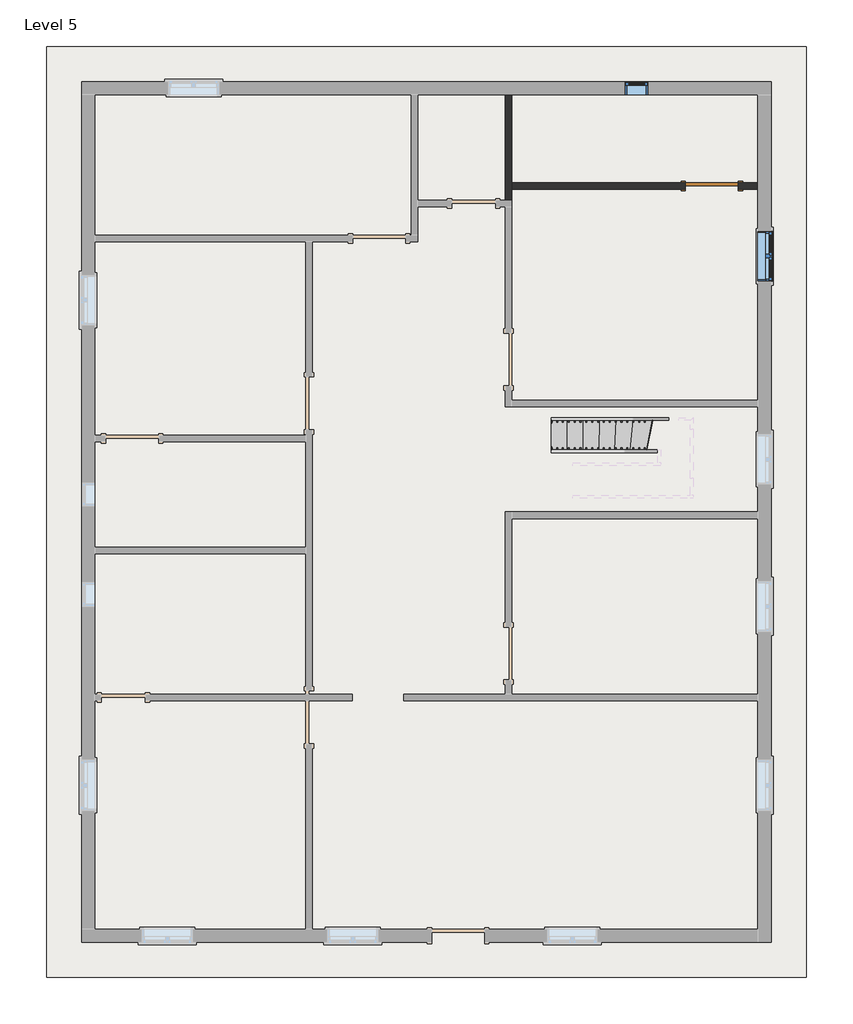
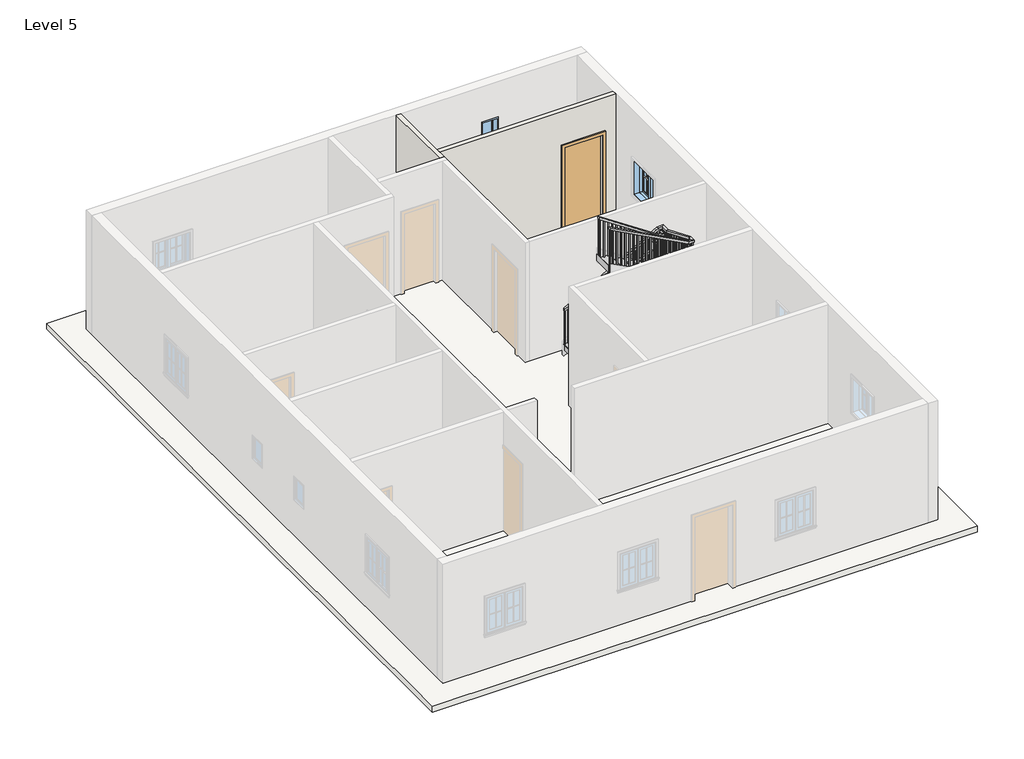
# One storey, part 2 of 3: 2 railings, 2 walls, 2 windows, 1 door, 1 roof, 1 stair flight.
"""IFC4 building model written with IfcOpenShell, lengths in millimetres."""

from ifc_helpers import new_model, si_unit, frame, origin, place, context, project, spatial, polyline, outline, extrude, faceted_brep, transform, mapped, element, save
from components import door_e5f9f3c4, stair_flight_0d7771ed, window_373d1f99, window_339605e1

model = new_model("IFC4")

# Units and contexts
model_context = context("Model", 3, world=origin())
ifc_project = project(units=[si_unit("LENGTHUNIT", "METRE", prefix="MILLI")], contexts=[model_context])

# Site, building, storey
site = spatial("IfcSite", under=ifc_project)
building = spatial("IfcBuilding", under=site)
storey = spatial("IfcBuildingStorey", under=building, Name="Level 5", Elevation=9601.2)

# Door
placement = place(None, origin())
door_shape = door_e5f9f3c4(model_context)
element("IfcDoor", 1, ObjectType="Single-Flush : 36\" x 84\"", at=placement, inside=storey, context=model_context, shape_type="MappedRepresentation", body=[
    mapped(door_shape, transform((3624.6756993, 7272.227558, 9601.2), x_axis=(1.0, 0.0, 0.0), y_axis=(0.0, 1.0, 0.0), z_axis=(0.0, 0.0, 1.0))),
])

# Railings
element("IfcRailing", 2, ObjectType="Handrail - Rectangular", at=placement, inside=storey, context=model_context, shape_type="SolidModel", body=[
    faceted_brep([(838.4202681, 2744.677558, 10854.2666667), (838.4202681, 2744.677558, 10793.9442501), (838.4202681, 2693.877558, 10793.9442501), (838.4202681, 2693.877558, 10854.2666667), (2663.2073911, 2744.677558, 12022.7510761), (2714.0073911, 2744.677558, 11994.9579377), (2714.0073911, 2693.877558, 11994.9579377), (2663.2073911, 2693.877558, 12022.7510761), (2663.2073911, 2744.677558, 12235.0070819), (2714.0073911, 2744.677558, 12184.2070819), (2714.0073911, 2693.877558, 12184.2070819), (2663.2073911, 2693.877558, 12235.0070819), (2790.2073911, 2744.677558, 12235.0070819), (2790.2073911, 2744.677558, 12184.2070819), (2739.4073911, 2693.877558, 12184.2070819), (2739.4073911, 2693.877558, 12235.0070819), (2790.2073911, 2617.677558, 12235.0070819), (2790.2073911, 2595.5706127, 12184.2070819), (2739.4073911, 2595.5706127, 12184.2070819), (2739.4073911, 2617.677558, 12235.0070819), (2790.2073911, 2490.677558, 12371.3650362), (2790.2073911, 2439.877558, 12351.3723294), (2739.4073911, 2439.877558, 12351.3723294), (2739.4073911, 2490.677558, 12371.3650362), (2790.2073911, 2490.677558, 12586.9137911), (2790.2073911, 2439.877558, 12536.1137911), (2739.4073911, 2439.877558, 12536.1137911), (2739.4073911, 2490.677558, 12586.9137911), (2790.2073911, 2363.677558, 12586.9137911), (2790.2073911, 2363.677558, 12536.1137911), (2739.4073911, 2414.477558, 12536.1137911), (2739.4073911, 2414.477558, 12586.9137911), (2663.2073911, 2363.677558, 12586.9137911), (2647.7076469, 2363.677558, 12536.1137911), (2647.7076469, 2414.477558, 12536.1137911), (2663.2073911, 2414.477558, 12586.9137911), (1211.6756993, 2363.677558, 13563.6), (1211.6756993, 2414.477558, 13563.6), (1211.6756993, 2414.477558, 13502.3707504), (1211.6756993, 2363.677558, 13502.3707504)], [[[0, 1, 2, 3]], [[1, 0, 4, 5]], [[2, 1, 5, 6]], [[3, 2, 6, 7]], [[0, 3, 7, 4]], [[5, 4, 8, 9]], [[6, 5, 9, 10]], [[7, 6, 10, 11]], [[4, 7, 11, 8]], [[9, 8, 12, 13]], [[10, 9, 13, 14]], [[11, 10, 14, 15]], [[8, 11, 15, 12]], [[13, 12, 16, 17]], [[14, 13, 17, 18]], [[15, 14, 18, 19]], [[12, 15, 19, 16]], [[17, 16, 20, 21]], [[18, 17, 21, 22]], [[19, 18, 22, 23]], [[16, 19, 23, 20]], [[21, 20, 24, 25]], [[22, 21, 25, 26]], [[23, 22, 26, 27]], [[20, 23, 27, 24]], [[25, 24, 28, 29]], [[26, 25, 29, 30]], [[27, 26, 30, 31]], [[24, 27, 31, 28]], [[29, 28, 32, 33]], [[30, 29, 33, 34]], [[31, 30, 34, 35]], [[28, 31, 35, 32]], [[36, 37, 38, 39]], [[33, 32, 36, 39]], [[34, 33, 39, 38]], [[35, 34, 38, 37]], [[32, 35, 37, 36]]]),
    extrude(outline(polyline([(13476.3599798, 1250.3323911), (13489.1780756, 1231.2823911), (12479.8666667, 1231.2823911), (12479.8666667, 1250.3323911), (13476.3599798, 1250.3323911)])), frame((0.0, 2379.552558, 0.0), z_axis=(0.0, 1.0, 0.0), x_axis=(0.0, 0.0, 1.0)), (0.0, 0.0, 1.0), 19.05),
    extrude(outline(polyline([(13407.9968022, 1351.9323911), (13420.814898, 1332.8823911), (12479.8666667, 1332.8823911), (12479.8666667, 1351.9323911), (13407.9968022, 1351.9323911)])), frame((0.0, 2379.552558, 0.0), z_axis=(0.0, 1.0, 0.0), x_axis=(0.0, 0.0, 1.0)), (0.0, 0.0, 1.0), 19.05),
    extrude(outline(polyline([(13339.6336246, 1453.5323911), (13352.4517204, 1434.4823911), (12479.8666667, 1434.4823911), (12479.8666667, 1453.5323911), (13339.6336246, 1453.5323911)])), frame((0.0, 2379.552558, 0.0), z_axis=(0.0, 1.0, 0.0), x_axis=(0.0, 0.0, 1.0)), (0.0, 0.0, 1.0), 19.05),
    extrude(outline(polyline([(13271.270447, 1555.1323911), (13284.0885428, 1536.0823911), (12310.5333333, 1536.0823911), (12310.5333333, 1555.1323911), (13271.270447, 1555.1323911)])), frame((0.0, 2379.552558, 0.0), z_axis=(0.0, 1.0, 0.0), x_axis=(0.0, 0.0, 1.0)), (0.0, 0.0, 1.0), 19.05),
    extrude(outline(polyline([(13202.9072694, 1656.7323911), (13215.7253652, 1637.6823911), (12310.5333333, 1637.6823911), (12310.5333333, 1656.7323911), (13202.9072694, 1656.7323911)])), frame((0.0, 2379.552558, 0.0), z_axis=(0.0, 1.0, 0.0), x_axis=(0.0, 0.0, 1.0)), (0.0, 0.0, 1.0), 19.05),
    extrude(outline(polyline([(13134.5440918, 1758.3323911), (13147.3621876, 1739.2823911), (12310.5333333, 1739.2823911), (12310.5333333, 1758.3323911), (13134.5440918, 1758.3323911)])), frame((0.0, 2379.552558, 0.0), z_axis=(0.0, 1.0, 0.0), x_axis=(0.0, 0.0, 1.0)), (0.0, 0.0, 1.0), 19.05),
    extrude(outline(polyline([(13066.1809143, 1859.9323911), (13078.9990101, 1840.8823911), (12141.2, 1840.8823911), (12141.2, 1859.9323911), (13066.1809143, 1859.9323911)])), frame((0.0, 2379.552558, 0.0), z_axis=(0.0, 1.0, 0.0), x_axis=(0.0, 0.0, 1.0)), (0.0, 0.0, 1.0), 19.05),
    extrude(outline(polyline([(12997.8177367, 1961.5323911), (13010.6358325, 1942.4823911), (12141.2, 1942.4823911), (12141.2, 1961.5323911), (12997.8177367, 1961.5323911)])), frame((0.0, 2379.552558, 0.0), z_axis=(0.0, 1.0, 0.0), x_axis=(0.0, 0.0, 1.0)), (0.0, 0.0, 1.0), 19.05),
    extrude(outline(polyline([(12929.4545591, 2063.1323911), (12942.2726549, 2044.0823911), (11971.8666667, 2044.0823911), (11971.8666667, 2063.1323911), (12929.4545591, 2063.1323911)])), frame((0.0, 2379.552558, 0.0), z_axis=(0.0, 1.0, 0.0), x_axis=(0.0, 0.0, 1.0)), (0.0, 0.0, 1.0), 19.05),
    extrude(outline(polyline([(12861.0913815, 2164.7323911), (12873.9094773, 2145.6823911), (11971.8666667, 2145.6823911), (11971.8666667, 2164.7323911), (12861.0913815, 2164.7323911)])), frame((0.0, 2379.552558, 0.0), z_axis=(0.0, 1.0, 0.0), x_axis=(0.0, 0.0, 1.0)), (0.0, 0.0, 1.0), 19.05),
    extrude(outline(polyline([(12792.7282039, 2266.3323911), (12805.5462997, 2247.2823911), (11971.8666667, 2247.2823911), (11971.8666667, 2266.3323911), (12792.7282039, 2266.3323911)])), frame((0.0, 2379.552558, 0.0), z_axis=(0.0, 1.0, 0.0), x_axis=(0.0, 0.0, 1.0)), (0.0, 0.0, 1.0), 19.05),
    extrude(outline(polyline([(12724.3650263, 2367.9323911), (12737.1831221, 2348.8823911), (11802.5333333, 2348.8823911), (11802.5333333, 2367.9323911), (12724.3650263, 2367.9323911)])), frame((0.0, 2379.552558, 0.0), z_axis=(0.0, 1.0, 0.0), x_axis=(0.0, 0.0, 1.0)), (0.0, 0.0, 1.0), 19.05),
    extrude(outline(polyline([(12656.0018487, 2469.5323911), (12668.8199445, 2450.4823911), (11802.5333333, 2450.4823911), (11802.5333333, 2469.5323911), (12656.0018487, 2469.5323911)])), frame((0.0, 2379.552558, 0.0), z_axis=(0.0, 1.0, 0.0), x_axis=(0.0, 0.0, 1.0)), (0.0, 0.0, 1.0), 19.05),
    extrude(outline(polyline([(12587.6386712, 2571.1323911), (12600.456767, 2552.0823911), (11633.2, 2552.0823911), (11633.2, 2571.1323911), (12587.6386712, 2571.1323911)])), frame((0.0, 2379.552558, 0.0), z_axis=(0.0, 1.0, 0.0), x_axis=(0.0, 0.0, 1.0)), (0.0, 0.0, 1.0), 19.05),
    extrude(outline(polyline([(12519.2754936, 2672.7323911), (12532.0935894, 2653.6823911), (11633.2, 2653.6823911), (11633.2, 2672.7323911), (12519.2754936, 2672.7323911)])), frame((0.0, 2379.552558, 0.0), z_axis=(0.0, 1.0, 0.0), x_axis=(0.0, 0.0, 1.0)), (0.0, 0.0, 1.0), 19.05),
    extrude(outline(polyline([(2755.2823911, 2424.002558), (2774.3323911, 2424.002558), (2774.3323911, 2404.952558), (2755.2823911, 2404.952558), (2755.2823911, 2424.002558)])), frame((0.0, 0.0, 11463.8666667), z_axis=(0.0, 0.0, 1.0), x_axis=(1.0, 0.0, 0.0)), (0.0, 0.0, 1.0), 1072.2471245),
    extrude(outline(polyline([(2506.552558, 12279.7844034), (2525.602558, 12259.3307103), (2525.602558, 11294.5333333), (2506.552558, 11294.5333333), (2506.552558, 12279.7844034)])), frame((2755.2823911, 0.0, 0.0), z_axis=(1.0, 0.0, 0.0), x_axis=(0.0, 1.0, 0.0)), (0.0, 0.0, 1.0), 19.05),
    extrude(outline(polyline([(2608.152558, 12170.69804), (2627.202558, 12150.2443468), (2627.202558, 11294.5333333), (2608.152558, 11294.5333333), (2608.152558, 12170.69804)])), frame((2755.2823911, 0.0, 0.0), z_axis=(1.0, 0.0, 0.0), x_axis=(0.0, 1.0, 0.0)), (0.0, 0.0, 1.0), 19.05),
    extrude(outline(polyline([(2657.6952681, 2709.752558), (2657.6952681, 2728.802558), (2676.7452681, 2728.802558), (2676.7452681, 2709.752558), (2657.6952681, 2709.752558)])), frame((0.0, 0.0, 10955.8666667), z_axis=(0.0, 0.0, 1.0), x_axis=(1.0, 0.0, 0.0)), (0.0, 0.0, 1.0), 1228.3404152),
    extrude(outline(polyline([(11906.0389489, 2575.1452681), (11893.8404695, 2556.0952681), (10955.8666667, 2556.0952681), (10955.8666667, 2575.1452681), (11906.0389489, 2575.1452681)])), frame((0.0, 2709.752558, 0.0), z_axis=(0.0, 1.0, 0.0), x_axis=(0.0, 0.0, 1.0)), (0.0, 0.0, 1.0), 19.05),
    extrude(outline(polyline([(11840.9803925, 2473.5452681), (11828.7819131, 2454.4952681), (10786.5333333, 2454.4952681), (10786.5333333, 2473.5452681), (11840.9803925, 2473.5452681)])), frame((0.0, 2709.752558, 0.0), z_axis=(0.0, 1.0, 0.0), x_axis=(0.0, 0.0, 1.0)), (0.0, 0.0, 1.0), 19.05),
    extrude(outline(polyline([(11775.921836, 2371.9452681), (11763.7233567, 2352.8952681), (10786.5333333, 2352.8952681), (10786.5333333, 2371.9452681), (11775.921836, 2371.9452681)])), frame((0.0, 2709.752558, 0.0), z_axis=(0.0, 1.0, 0.0), x_axis=(0.0, 0.0, 1.0)), (0.0, 0.0, 1.0), 19.05),
    extrude(outline(polyline([(11710.8632796, 2270.3452681), (11698.6648003, 2251.2952681), (10786.5333333, 2251.2952681), (10786.5333333, 2270.3452681), (11710.8632796, 2270.3452681)])), frame((0.0, 2709.752558, 0.0), z_axis=(0.0, 1.0, 0.0), x_axis=(0.0, 0.0, 1.0)), (0.0, 0.0, 1.0), 19.05),
    extrude(outline(polyline([(11645.8047232, 2168.7452681), (11633.6062439, 2149.6952681), (10617.2, 2149.6952681), (10617.2, 2168.7452681), (11645.8047232, 2168.7452681)])), frame((0.0, 2709.752558, 0.0), z_axis=(0.0, 1.0, 0.0), x_axis=(0.0, 0.0, 1.0)), (0.0, 0.0, 1.0), 19.05),
    extrude(outline(polyline([(11580.7461668, 2067.1452681), (11568.5476875, 2048.0952681), (10617.2, 2048.0952681), (10617.2, 2067.1452681), (11580.7461668, 2067.1452681)])), frame((0.0, 2709.752558, 0.0), z_axis=(0.0, 1.0, 0.0), x_axis=(0.0, 0.0, 1.0)), (0.0, 0.0, 1.0), 19.05),
    extrude(outline(polyline([(11515.6876104, 1965.5452681), (11503.489131, 1946.4952681), (10617.2, 1946.4952681), (10617.2, 1965.5452681), (11515.6876104, 1965.5452681)])), frame((0.0, 2709.752558, 0.0), z_axis=(0.0, 1.0, 0.0), x_axis=(0.0, 0.0, 1.0)), (0.0, 0.0, 1.0), 19.05),
    extrude(outline(polyline([(11450.6290539, 1863.9452681), (11438.4305746, 1844.8952681), (10447.8666667, 1844.8952681), (10447.8666667, 1863.9452681), (11450.6290539, 1863.9452681)])), frame((0.0, 2709.752558, 0.0), z_axis=(0.0, 1.0, 0.0), x_axis=(0.0, 0.0, 1.0)), (0.0, 0.0, 1.0), 19.05),
    extrude(outline(polyline([(11385.5704975, 1762.3452681), (11373.3720182, 1743.2952681), (10447.8666667, 1743.2952681), (10447.8666667, 1762.3452681), (11385.5704975, 1762.3452681)])), frame((0.0, 2709.752558, 0.0), z_axis=(0.0, 1.0, 0.0), x_axis=(0.0, 0.0, 1.0)), (0.0, 0.0, 1.0), 19.05),
    extrude(outline(polyline([(11320.5119411, 1660.7452681), (11308.3134618, 1641.6952681), (10278.5333333, 1641.6952681), (10278.5333333, 1660.7452681), (11320.5119411, 1660.7452681)])), frame((0.0, 2709.752558, 0.0), z_axis=(0.0, 1.0, 0.0), x_axis=(0.0, 0.0, 1.0)), (0.0, 0.0, 1.0), 19.05),
    extrude(outline(polyline([(11255.4533847, 1559.1452681), (11243.2549054, 1540.0952681), (10278.5333333, 1540.0952681), (10278.5333333, 1559.1452681), (11255.4533847, 1559.1452681)])), frame((0.0, 2709.752558, 0.0), z_axis=(0.0, 1.0, 0.0), x_axis=(0.0, 0.0, 1.0)), (0.0, 0.0, 1.0), 19.05),
    extrude(outline(polyline([(11190.3948283, 1457.5452681), (11178.1963489, 1438.4952681), (10278.5333333, 1438.4952681), (10278.5333333, 1457.5452681), (11190.3948283, 1457.5452681)])), frame((0.0, 2709.752558, 0.0), z_axis=(0.0, 1.0, 0.0), x_axis=(0.0, 0.0, 1.0)), (0.0, 0.0, 1.0), 19.05),
    extrude(outline(polyline([(11125.3362719, 1355.9452681), (11113.1377925, 1336.8952681), (10109.2, 1336.8952681), (10109.2, 1355.9452681), (11125.3362719, 1355.9452681)])), frame((0.0, 2709.752558, 0.0), z_axis=(0.0, 1.0, 0.0), x_axis=(0.0, 0.0, 1.0)), (0.0, 0.0, 1.0), 19.05),
    extrude(outline(polyline([(11060.2777154, 1254.3452681), (11048.0792361, 1235.2952681), (10109.2, 1235.2952681), (10109.2, 1254.3452681), (11060.2777154, 1254.3452681)])), frame((0.0, 2709.752558, 0.0), z_axis=(0.0, 1.0, 0.0), x_axis=(0.0, 0.0, 1.0)), (0.0, 0.0, 1.0), 19.05),
    extrude(outline(polyline([(10995.219159, 1152.7452681), (10983.0206797, 1133.6952681), (10109.2, 1133.6952681), (10109.2, 1152.7452681), (10995.219159, 1152.7452681)])), frame((0.0, 2709.752558, 0.0), z_axis=(0.0, 1.0, 0.0), x_axis=(0.0, 0.0, 1.0)), (0.0, 0.0, 1.0), 19.05),
    extrude(outline(polyline([(10930.1606026, 1051.1452681), (10917.9621233, 1032.0952681), (9939.8666667, 1032.0952681), (9939.8666667, 1051.1452681), (10930.1606026, 1051.1452681)])), frame((0.0, 2709.752558, 0.0), z_axis=(0.0, 1.0, 0.0), x_axis=(0.0, 0.0, 1.0)), (0.0, 0.0, 1.0), 19.05),
    extrude(outline(polyline([(10865.1020462, 949.5452681), (10852.9035669, 930.4952681), (9939.8666667, 930.4952681), (9939.8666667, 949.5452681), (10865.1020462, 949.5452681)])), frame((0.0, 2709.752558, 0.0), z_axis=(0.0, 1.0, 0.0), x_axis=(0.0, 0.0, 1.0)), (0.0, 0.0, 1.0), 19.05),
    extrude(outline(polyline([(2755.2823911, 2398.602558), (2774.3323911, 2398.602558), (2774.3323911, 2379.552558), (2755.2823911, 2379.552558), (2755.2823911, 2398.602558)])), frame((0.0, 0.0, 11463.8666667), z_axis=(0.0, 0.0, 1.0), x_axis=(1.0, 0.0, 0.0)), (0.0, 0.0, 1.0), 1072.2471245),
    extrude(outline(polyline([(2755.2823911, 2709.752558), (2755.2823911, 2728.802558), (2774.3323911, 2728.802558), (2774.3323911, 2709.752558), (2755.2823911, 2709.752558)])), frame((0.0, 0.0, 11125.2), z_axis=(0.0, 0.0, 1.0), x_axis=(1.0, 0.0, 0.0)), (0.0, 0.0, 1.0), 1059.0070819),
    extrude(outline(polyline([(13489.5526546, 1230.7256993), (13502.3707504, 1211.6756993), (12479.8666667, 1211.6756993), (12479.8666667, 1230.7256993), (13489.5526546, 1230.7256993)])), frame((0.0, 2379.552558, 0.0), z_axis=(0.0, 1.0, 0.0), x_axis=(0.0, 0.0, 1.0)), (0.0, 0.0, 1.0), 19.05),
    extrude(outline(polyline([(10806.1427294, 857.4702681), (10793.9442501, 838.4202681), (9939.8666667, 838.4202681), (9939.8666667, 857.4702681), (10806.1427294, 857.4702681)])), frame((0.0, 2709.752558, 0.0), z_axis=(0.0, 1.0, 0.0), x_axis=(0.0, 0.0, 1.0)), (0.0, 0.0, 1.0), 19.05),
])
element("IfcRailing", 3, ObjectType="Handrail - Rectangular", at=placement, inside=storey, context=model_context, shape_type="SolidModel", body=[
    faceted_brep([(838.4202681, 3202.4524989, 10854.2666667), (838.4202681, 3202.4524989, 10795.6953096), (838.4202681, 3151.6524989, 10795.6953096), (838.4202681, 3151.6524989, 10854.2666667), (3089.9785641, 3202.4524989, 12146.4368493), (3103.5198636, 3202.4524989, 12095.6368493), (3103.5198636, 3151.6524989, 12095.6368493), (3089.9785641, 3151.6524989, 12146.4368493), (3247.982332, 3202.4524989, 12146.4368493), (3247.982332, 3202.4524989, 12095.6368493), (3197.182332, 3151.6524989, 12095.6368493), (3197.182332, 3151.6524989, 12146.4368493), (3247.982332, 2995.1725832, 12146.4368493), (3247.982332, 2984.9732412, 12095.6368493), (3197.182332, 2984.9732412, 12095.6368493), (3197.182332, 2995.1725832, 12146.4368493), (3247.982332, 2050.6126885, 12541.6552365), (3247.982332, 2040.4133465, 12490.8552365), (3197.182332, 2040.4133465, 12490.8552365), (3197.182332, 2050.6126885, 12541.6552365), (3247.982332, 1905.9026171, 12541.6552365), (3247.982332, 1905.9026171, 12490.8552365), (3197.182332, 1956.7026171, 12490.8552365), (3197.182332, 1956.7026171, 12541.6552365), (3128.9262072, 1905.9026171, 12541.6552365), (3116.2326609, 1905.9026171, 12490.8552365), (3116.2326609, 1956.7026171, 12490.8552365), (3128.9262072, 1956.7026171, 12541.6552365), (1211.6756993, 1905.9026171, 13563.6), (1211.6756993, 1956.7026171, 13563.6), (1211.6756993, 1956.7026171, 13506.0340072), (1211.6756993, 1905.9026171, 13506.0340072)], [[[0, 1, 2, 3]], [[1, 0, 4, 5]], [[2, 1, 5, 6]], [[3, 2, 6, 7]], [[0, 3, 7, 4]], [[5, 4, 8, 9]], [[6, 5, 9, 10]], [[7, 6, 10, 11]], [[4, 7, 11, 8]], [[9, 8, 12, 13]], [[10, 9, 13, 14]], [[11, 10, 14, 15]], [[8, 11, 15, 12]], [[13, 12, 16, 17]], [[14, 13, 17, 18]], [[15, 14, 18, 19]], [[12, 15, 19, 16]], [[17, 16, 20, 21]], [[18, 17, 21, 22]], [[19, 18, 22, 23]], [[16, 19, 23, 20]], [[21, 20, 24, 25]], [[22, 21, 25, 26]], [[23, 22, 26, 27]], [[20, 23, 27, 24]], [[28, 29, 30, 31]], [[25, 24, 28, 31]], [[26, 25, 31, 30]], [[27, 26, 30, 29]], [[24, 27, 29, 28]]]),
    extrude(outline(polyline([(13468.1989368, 1282.657332), (12479.8666667, 1282.657332), (12479.8666667, 1301.707332), (13458.0447876, 1301.707332), (13468.1989368, 1282.657332)])), frame((0.0, 1921.7776171, 0.0), z_axis=(0.0, 1.0, 0.0), x_axis=(0.0, 0.0, 1.0)), (0.0, 0.0, 1.0), 19.05),
    extrude(outline(polyline([(13414.0434743, 1384.257332), (12479.8666667, 1384.257332), (12479.8666667, 1403.307332), (13403.8893251, 1403.307332), (13414.0434743, 1384.257332)])), frame((0.0, 1921.7776171, 0.0), z_axis=(0.0, 1.0, 0.0), x_axis=(0.0, 0.0, 1.0)), (0.0, 0.0, 1.0), 19.05),
    extrude(outline(polyline([(13359.8880118, 1485.857332), (12310.5333333, 1485.857332), (12310.5333333, 1504.907332), (13349.7338626, 1504.907332), (13359.8880118, 1485.857332)])), frame((0.0, 1921.7776171, 0.0), z_axis=(0.0, 1.0, 0.0), x_axis=(0.0, 0.0, 1.0)), (0.0, 0.0, 1.0), 19.05),
    extrude(outline(polyline([(13305.7325493, 1587.457332), (12310.5333333, 1587.457332), (12310.5333333, 1606.507332), (13295.5784001, 1606.507332), (13305.7325493, 1587.457332)])), frame((0.0, 1921.7776171, 0.0), z_axis=(0.0, 1.0, 0.0), x_axis=(0.0, 0.0, 1.0)), (0.0, 0.0, 1.0), 19.05),
    extrude(outline(polyline([(13251.5770868, 1689.057332), (12310.5333333, 1689.057332), (12310.5333333, 1708.107332), (13241.4229376, 1708.107332), (13251.5770868, 1689.057332)])), frame((0.0, 1921.7776171, 0.0), z_axis=(0.0, 1.0, 0.0), x_axis=(0.0, 0.0, 1.0)), (0.0, 0.0, 1.0), 19.05),
    extrude(outline(polyline([(13197.4216243, 1790.657332), (12141.2, 1790.657332), (12141.2, 1809.707332), (13187.2674751, 1809.707332), (13197.4216243, 1790.657332)])), frame((0.0, 1921.7776171, 0.0), z_axis=(0.0, 1.0, 0.0), x_axis=(0.0, 0.0, 1.0)), (0.0, 0.0, 1.0), 19.05),
    extrude(outline(polyline([(13143.2661618, 1892.257332), (12141.2, 1892.257332), (12141.2, 1911.307332), (13133.1120126, 1911.307332), (13143.2661618, 1892.257332)])), frame((0.0, 1921.7776171, 0.0), z_axis=(0.0, 1.0, 0.0), x_axis=(0.0, 0.0, 1.0)), (0.0, 0.0, 1.0), 19.05),
    extrude(outline(polyline([(13089.1106993, 1993.857332), (12141.2, 1993.857332), (12141.2, 2012.907332), (13078.9565501, 2012.907332), (13089.1106993, 1993.857332)])), frame((0.0, 1921.7776171, 0.0), z_axis=(0.0, 1.0, 0.0), x_axis=(0.0, 0.0, 1.0)), (0.0, 0.0, 1.0), 19.05),
    extrude(outline(polyline([(13034.9552369, 2095.457332), (11971.8666667, 2095.457332), (11971.8666667, 2114.507332), (13024.8010876, 2114.507332), (13034.9552369, 2095.457332)])), frame((0.0, 1921.7776171, 0.0), z_axis=(0.0, 1.0, 0.0), x_axis=(0.0, 0.0, 1.0)), (0.0, 0.0, 1.0), 19.05),
    extrude(outline(polyline([(12980.7997744, 2197.057332), (11971.8666667, 2197.057332), (11971.8666667, 2216.107332), (12970.6456251, 2216.107332), (12980.7997744, 2197.057332)])), frame((0.0, 1921.7776171, 0.0), z_axis=(0.0, 1.0, 0.0), x_axis=(0.0, 0.0, 1.0)), (0.0, 0.0, 1.0), 19.05),
    extrude(outline(polyline([(12926.6443119, 2298.657332), (11971.8666667, 2298.657332), (11971.8666667, 2317.707332), (12916.4901626, 2317.707332), (12926.6443119, 2298.657332)])), frame((0.0, 1921.7776171, 0.0), z_axis=(0.0, 1.0, 0.0), x_axis=(0.0, 0.0, 1.0)), (0.0, 0.0, 1.0), 19.05),
    extrude(outline(polyline([(12872.4888494, 2400.257332), (11802.5333333, 2400.257332), (11802.5333333, 2419.307332), (12862.3347002, 2419.307332), (12872.4888494, 2400.257332)])), frame((0.0, 1921.7776171, 0.0), z_axis=(0.0, 1.0, 0.0), x_axis=(0.0, 0.0, 1.0)), (0.0, 0.0, 1.0), 19.05),
    extrude(outline(polyline([(12818.3333869, 2501.857332), (11802.5333333, 2501.857332), (11802.5333333, 2520.907332), (12808.1792377, 2520.907332), (12818.3333869, 2501.857332)])), frame((0.0, 1921.7776171, 0.0), z_axis=(0.0, 1.0, 0.0), x_axis=(0.0, 0.0, 1.0)), (0.0, 0.0, 1.0), 19.05),
    extrude(outline(polyline([(12764.1779244, 2603.457332), (11802.5333333, 2603.457332), (11802.5333333, 2622.507332), (12754.0237752, 2622.507332), (12764.1779244, 2603.457332)])), frame((0.0, 1921.7776171, 0.0), z_axis=(0.0, 1.0, 0.0), x_axis=(0.0, 0.0, 1.0)), (0.0, 0.0, 1.0), 19.05),
    extrude(outline(polyline([(12710.0224619, 2705.057332), (11633.2, 2705.057332), (11633.2, 2724.107332), (12699.8683127, 2724.107332), (12710.0224619, 2705.057332)])), frame((0.0, 1921.7776171, 0.0), z_axis=(0.0, 1.0, 0.0), x_axis=(0.0, 0.0, 1.0)), (0.0, 0.0, 1.0), 19.05),
    extrude(outline(polyline([(12655.8669994, 2806.657332), (11633.2, 2806.657332), (11633.2, 2825.707332), (12645.7128502, 2825.707332), (12655.8669994, 2806.657332)])), frame((0.0, 1921.7776171, 0.0), z_axis=(0.0, 1.0, 0.0), x_axis=(0.0, 0.0, 1.0)), (0.0, 0.0, 1.0), 19.05),
    extrude(outline(polyline([(12601.7115369, 2908.257332), (11633.2, 2908.257332), (11633.2, 2927.307332), (12591.5573877, 2927.307332), (12601.7115369, 2908.257332)])), frame((0.0, 1921.7776171, 0.0), z_axis=(0.0, 1.0, 0.0), x_axis=(0.0, 0.0, 1.0)), (0.0, 0.0, 1.0), 19.05),
    extrude(outline(polyline([(12547.5560744, 3009.857332), (11633.2, 3009.857332), (11633.2, 3028.907332), (12537.4019252, 3028.907332), (12547.5560744, 3009.857332)])), frame((0.0, 1921.7776171, 0.0), z_axis=(0.0, 1.0, 0.0), x_axis=(0.0, 0.0, 1.0)), (0.0, 0.0, 1.0), 19.05),
    extrude(outline(polyline([(12493.4006119, 3111.457332), (11463.8666667, 3111.457332), (11463.8666667, 3130.507332), (12483.2464627, 3130.507332), (12493.4006119, 3111.457332)])), frame((0.0, 1921.7776171, 0.0), z_axis=(0.0, 1.0, 0.0), x_axis=(0.0, 0.0, 1.0)), (0.0, 0.0, 1.0), 19.05),
    extrude(outline(polyline([(3232.107332, 1967.3774989), (3232.107332, 1948.3274989), (3213.057332, 1948.3274989), (3213.057332, 1967.3774989), (3232.107332, 1967.3774989)])), frame((0.0, 0.0, 11463.8666667), z_axis=(0.0, 0.0, 1.0), x_axis=(1.0, 0.0, 0.0)), (0.0, 0.0, 1.0), 1026.9885698),
    extrude(outline(polyline([(2068.9774989, 12478.9035558), (2068.9774989, 11463.8666667), (2049.9274989, 11463.8666667), (2049.9274989, 12486.8743688), (2068.9774989, 12478.9035558)])), frame((3213.057332, 0.0, 0.0), z_axis=(1.0, 0.0, 0.0), x_axis=(0.0, 1.0, 0.0)), (0.0, 0.0, 1.0), 19.05),
    extrude(outline(polyline([(2170.5774989, 12436.3925532), (2170.5774989, 11463.8666667), (2151.5274989, 11463.8666667), (2151.5274989, 12444.3633662), (2170.5774989, 12436.3925532)])), frame((3213.057332, 0.0, 0.0), z_axis=(1.0, 0.0, 0.0), x_axis=(0.0, 1.0, 0.0)), (0.0, 0.0, 1.0), 19.05),
    extrude(outline(polyline([(2272.1774989, 12393.8815506), (2272.1774989, 11463.8666667), (2253.1274989, 11463.8666667), (2253.1274989, 12401.8523636), (2272.1774989, 12393.8815506)])), frame((3213.057332, 0.0, 0.0), z_axis=(1.0, 0.0, 0.0), x_axis=(0.0, 1.0, 0.0)), (0.0, 0.0, 1.0), 19.05),
    extrude(outline(polyline([(2373.7774989, 12351.370548), (2373.7774989, 11463.8666667), (2354.7274989, 11463.8666667), (2354.7274989, 12359.341361), (2373.7774989, 12351.370548)])), frame((3213.057332, 0.0, 0.0), z_axis=(1.0, 0.0, 0.0), x_axis=(0.0, 1.0, 0.0)), (0.0, 0.0, 1.0), 19.05),
    extrude(outline(polyline([(2475.3774989, 12308.8595454), (2475.3774989, 11294.5333333), (2456.3274989, 11294.5333333), (2456.3274989, 12316.8303584), (2475.3774989, 12308.8595454)])), frame((3213.057332, 0.0, 0.0), z_axis=(1.0, 0.0, 0.0), x_axis=(0.0, 1.0, 0.0)), (0.0, 0.0, 1.0), 19.05),
    extrude(outline(polyline([(2576.9774989, 12266.3485428), (2576.9774989, 11294.5333333), (2557.9274989, 11294.5333333), (2557.9274989, 12274.3193558), (2576.9774989, 12266.3485428)])), frame((3213.057332, 0.0, 0.0), z_axis=(1.0, 0.0, 0.0), x_axis=(0.0, 1.0, 0.0)), (0.0, 0.0, 1.0), 19.05),
    extrude(outline(polyline([(2678.5774989, 12223.8375402), (2678.5774989, 11294.5333333), (2659.5274989, 11294.5333333), (2659.5274989, 12231.8083532), (2678.5774989, 12223.8375402)])), frame((3213.057332, 0.0, 0.0), z_axis=(1.0, 0.0, 0.0), x_axis=(0.0, 1.0, 0.0)), (0.0, 0.0, 1.0), 19.05),
    extrude(outline(polyline([(2780.1774989, 12181.3265376), (2780.1774989, 11294.5333333), (2761.1274989, 11294.5333333), (2761.1274989, 12189.2973506), (2780.1774989, 12181.3265376)])), frame((3213.057332, 0.0, 0.0), z_axis=(1.0, 0.0, 0.0), x_axis=(0.0, 1.0, 0.0)), (0.0, 0.0, 1.0), 19.05),
    extrude(outline(polyline([(2881.7774989, 12138.815535), (2881.7774989, 11125.2), (2862.7274989, 11125.2), (2862.7274989, 12146.786348), (2881.7774989, 12138.815535)])), frame((3213.057332, 0.0, 0.0), z_axis=(1.0, 0.0, 0.0), x_axis=(0.0, 1.0, 0.0)), (0.0, 0.0, 1.0), 19.05),
    extrude(outline(polyline([(2983.3774989, 12096.3045324), (2983.3774989, 11125.2), (2964.3274989, 11125.2), (2964.3274989, 12104.2753454), (2983.3774989, 12096.3045324)])), frame((3213.057332, 0.0, 0.0), z_axis=(1.0, 0.0, 0.0), x_axis=(0.0, 1.0, 0.0)), (0.0, 0.0, 1.0), 19.05),
    extrude(outline(polyline([(3232.107332, 3084.9774989), (3232.107332, 3065.9274989), (3213.057332, 3065.9274989), (3213.057332, 3084.9774989), (3232.107332, 3084.9774989)])), frame((0.0, 0.0, 11125.2), z_axis=(0.0, 0.0, 1.0), x_axis=(1.0, 0.0, 0.0)), (0.0, 0.0, 1.0), 970.4368493),
    extrude(outline(polyline([(3165.6952681, 3186.5774989), (3184.7452681, 3186.5774989), (3184.7452681, 3167.5274989), (3165.6952681, 3167.5274989), (3165.6952681, 3186.5774989)])), frame((0.0, 0.0, 11125.2), z_axis=(0.0, 0.0, 1.0), x_axis=(1.0, 0.0, 0.0)), (0.0, 0.0, 1.0), 970.4368493),
    extrude(outline(polyline([(12073.0110585, 3064.0952681), (11125.2, 3064.0952681), (11125.2, 3083.1452681), (12083.943861, 3083.1452681), (12073.0110585, 3064.0952681)])), frame((0.0, 3167.5274989, 0.0), z_axis=(0.0, 1.0, 0.0), x_axis=(0.0, 0.0, 1.0)), (0.0, 0.0, 1.0), 19.05),
    extrude(outline(polyline([(12014.702779, 2962.4952681), (11125.2, 2962.4952681), (11125.2, 2981.5452681), (12025.6355814, 2981.5452681), (12014.702779, 2962.4952681)])), frame((0.0, 3167.5274989, 0.0), z_axis=(0.0, 1.0, 0.0), x_axis=(0.0, 0.0, 1.0)), (0.0, 0.0, 1.0), 19.05),
    extrude(outline(polyline([(11956.3944994, 2860.8952681), (10955.8666667, 2860.8952681), (10955.8666667, 2879.9452681), (11967.3273019, 2879.9452681), (11956.3944994, 2860.8952681)])), frame((0.0, 3167.5274989, 0.0), z_axis=(0.0, 1.0, 0.0), x_axis=(0.0, 0.0, 1.0)), (0.0, 0.0, 1.0), 19.05),
    extrude(outline(polyline([(11898.0862199, 2759.2952681), (10955.8666667, 2759.2952681), (10955.8666667, 2778.3452681), (11909.0190223, 2778.3452681), (11898.0862199, 2759.2952681)])), frame((0.0, 3167.5274989, 0.0), z_axis=(0.0, 1.0, 0.0), x_axis=(0.0, 0.0, 1.0)), (0.0, 0.0, 1.0), 19.05),
    extrude(outline(polyline([(11839.7779403, 2657.6952681), (10955.8666667, 2657.6952681), (10955.8666667, 2676.7452681), (11850.7107428, 2676.7452681), (11839.7779403, 2657.6952681)])), frame((0.0, 3167.5274989, 0.0), z_axis=(0.0, 1.0, 0.0), x_axis=(0.0, 0.0, 1.0)), (0.0, 0.0, 1.0), 19.05),
    extrude(outline(polyline([(11781.4696608, 2556.0952681), (10955.8666667, 2556.0952681), (10955.8666667, 2575.1452681), (11792.4024632, 2575.1452681), (11781.4696608, 2556.0952681)])), frame((0.0, 3167.5274989, 0.0), z_axis=(0.0, 1.0, 0.0), x_axis=(0.0, 0.0, 1.0)), (0.0, 0.0, 1.0), 19.05),
    extrude(outline(polyline([(11723.1613812, 2454.4952681), (10786.5333333, 2454.4952681), (10786.5333333, 2473.5452681), (11734.0941837, 2473.5452681), (11723.1613812, 2454.4952681)])), frame((0.0, 3167.5274989, 0.0), z_axis=(0.0, 1.0, 0.0), x_axis=(0.0, 0.0, 1.0)), (0.0, 0.0, 1.0), 19.05),
    extrude(outline(polyline([(11664.8531017, 2352.8952681), (10786.5333333, 2352.8952681), (10786.5333333, 2371.9452681), (11675.7859041, 2371.9452681), (11664.8531017, 2352.8952681)])), frame((0.0, 3167.5274989, 0.0), z_axis=(0.0, 1.0, 0.0), x_axis=(0.0, 0.0, 1.0)), (0.0, 0.0, 1.0), 19.05),
    extrude(outline(polyline([(11606.5448221, 2251.2952681), (10786.5333333, 2251.2952681), (10786.5333333, 2270.3452681), (11617.4776245, 2270.3452681), (11606.5448221, 2251.2952681)])), frame((0.0, 3167.5274989, 0.0), z_axis=(0.0, 1.0, 0.0), x_axis=(0.0, 0.0, 1.0)), (0.0, 0.0, 1.0), 19.05),
    extrude(outline(polyline([(11548.2365426, 2149.6952681), (10617.2, 2149.6952681), (10617.2, 2168.7452681), (11559.169345, 2168.7452681), (11548.2365426, 2149.6952681)])), frame((0.0, 3167.5274989, 0.0), z_axis=(0.0, 1.0, 0.0), x_axis=(0.0, 0.0, 1.0)), (0.0, 0.0, 1.0), 19.05),
    extrude(outline(polyline([(11489.928263, 2048.0952681), (10617.2, 2048.0952681), (10617.2, 2067.1452681), (11500.8610654, 2067.1452681), (11489.928263, 2048.0952681)])), frame((0.0, 3167.5274989, 0.0), z_axis=(0.0, 1.0, 0.0), x_axis=(0.0, 0.0, 1.0)), (0.0, 0.0, 1.0), 19.05),
    extrude(outline(polyline([(11431.6199835, 1946.4952681), (10447.8666667, 1946.4952681), (10447.8666667, 1965.5452681), (11442.5527859, 1965.5452681), (11431.6199835, 1946.4952681)])), frame((0.0, 3167.5274989, 0.0), z_axis=(0.0, 1.0, 0.0), x_axis=(0.0, 0.0, 1.0)), (0.0, 0.0, 1.0), 19.05),
    extrude(outline(polyline([(11373.3117039, 1844.8952681), (10447.8666667, 1844.8952681), (10447.8666667, 1863.9452681), (11384.2445063, 1863.9452681), (11373.3117039, 1844.8952681)])), frame((0.0, 3167.5274989, 0.0), z_axis=(0.0, 1.0, 0.0), x_axis=(0.0, 0.0, 1.0)), (0.0, 0.0, 1.0), 19.05),
    extrude(outline(polyline([(11315.0034244, 1743.2952681), (10447.8666667, 1743.2952681), (10447.8666667, 1762.3452681), (11325.9362268, 1762.3452681), (11315.0034244, 1743.2952681)])), frame((0.0, 3167.5274989, 0.0), z_axis=(0.0, 1.0, 0.0), x_axis=(0.0, 0.0, 1.0)), (0.0, 0.0, 1.0), 19.05),
    extrude(outline(polyline([(11256.6951448, 1641.6952681), (10278.5333333, 1641.6952681), (10278.5333333, 1660.7452681), (11267.6279472, 1660.7452681), (11256.6951448, 1641.6952681)])), frame((0.0, 3167.5274989, 0.0), z_axis=(0.0, 1.0, 0.0), x_axis=(0.0, 0.0, 1.0)), (0.0, 0.0, 1.0), 19.05),
    extrude(outline(polyline([(11198.3868653, 1540.0952681), (10278.5333333, 1540.0952681), (10278.5333333, 1559.1452681), (11209.3196677, 1559.1452681), (11198.3868653, 1540.0952681)])), frame((0.0, 3167.5274989, 0.0), z_axis=(0.0, 1.0, 0.0), x_axis=(0.0, 0.0, 1.0)), (0.0, 0.0, 1.0), 19.05),
    extrude(outline(polyline([(11140.0785857, 1438.4952681), (10278.5333333, 1438.4952681), (10278.5333333, 1457.5452681), (11151.0113881, 1457.5452681), (11140.0785857, 1438.4952681)])), frame((0.0, 3167.5274989, 0.0), z_axis=(0.0, 1.0, 0.0), x_axis=(0.0, 0.0, 1.0)), (0.0, 0.0, 1.0), 19.05),
    extrude(outline(polyline([(11081.7703062, 1336.8952681), (10109.2, 1336.8952681), (10109.2, 1355.9452681), (11092.7031086, 1355.9452681), (11081.7703062, 1336.8952681)])), frame((0.0, 3167.5274989, 0.0), z_axis=(0.0, 1.0, 0.0), x_axis=(0.0, 0.0, 1.0)), (0.0, 0.0, 1.0), 19.05),
    extrude(outline(polyline([(11023.4620266, 1235.2952681), (10109.2, 1235.2952681), (10109.2, 1254.3452681), (11034.394829, 1254.3452681), (11023.4620266, 1235.2952681)])), frame((0.0, 3167.5274989, 0.0), z_axis=(0.0, 1.0, 0.0), x_axis=(0.0, 0.0, 1.0)), (0.0, 0.0, 1.0), 19.05),
    extrude(outline(polyline([(10965.028643, 1133.6952681), (10109.2, 1133.6952681), (10109.2, 1152.7452681), (10975.9614454, 1152.7452681), (10965.028643, 1133.6952681)])), frame((0.0, 3167.5274989, 0.0), z_axis=(0.0, 1.0, 0.0), x_axis=(0.0, 0.0, 1.0)), (0.0, 0.0, 1.0), 19.05),
    extrude(outline(polyline([(10906.8454675, 1032.0952681), (9939.8666667, 1032.0952681), (9939.8666667, 1051.1452681), (10917.7782699, 1051.1452681), (10906.8454675, 1032.0952681)])), frame((0.0, 3167.5274989, 0.0), z_axis=(0.0, 1.0, 0.0), x_axis=(0.0, 0.0, 1.0)), (0.0, 0.0, 1.0), 19.05),
    extrude(outline(polyline([(10848.537188, 930.4952681), (9939.8666667, 930.4952681), (9939.8666667, 949.5452681), (10859.4699904, 949.5452681), (10848.537188, 930.4952681)])), frame((0.0, 3167.5274989, 0.0), z_axis=(0.0, 1.0, 0.0), x_axis=(0.0, 0.0, 1.0)), (0.0, 0.0, 1.0), 19.05),
    extrude(outline(polyline([(3232.107332, 1940.8276171), (3232.107332, 1921.7776171), (3213.057332, 1921.7776171), (3213.057332, 1940.8276171), (3232.107332, 1940.8276171)])), frame((0.0, 0.0, 11463.8666667), z_axis=(0.0, 0.0, 1.0), x_axis=(1.0, 0.0, 0.0)), (0.0, 0.0, 1.0), 1026.9885698),
    extrude(outline(polyline([(3213.057332, 3186.5774989), (3232.107332, 3186.5774989), (3232.107332, 3167.5274989), (3213.057332, 3167.5274989), (3213.057332, 3186.5774989)])), frame((0.0, 0.0, 11125.2), z_axis=(0.0, 0.0, 1.0), x_axis=(1.0, 0.0, 0.0)), (0.0, 0.0, 1.0), 970.4368493),
    extrude(outline(polyline([(13506.0340072, 1211.6756993), (12479.8666667, 1211.6756993), (12479.8666667, 1230.7256993), (13495.879858, 1230.7256993), (13506.0340072, 1211.6756993)])), frame((0.0, 1921.7776171, 0.0), z_axis=(0.0, 1.0, 0.0), x_axis=(0.0, 0.0, 1.0)), (0.0, 0.0, 1.0), 19.05),
    extrude(outline(polyline([(10795.6953096, 838.4202681), (9939.8666667, 838.4202681), (9939.8666667, 857.4702681), (10806.628112, 857.4702681), (10795.6953096, 838.4202681)])), frame((0.0, 3167.5274989, 0.0), z_axis=(0.0, 1.0, 0.0), x_axis=(0.0, 0.0, 1.0)), (0.0, 0.0, 1.0), 19.05),
])

# Roof
element("IfcRoof", 4, ObjectType="Generic - 12\"", at=placement, inside=storey, context=model_context, shape_type="SweptSolid", body=[
    extrude(outline(polyline([(-7919.6243007, 9691.577558), (5262.9756993, 9691.577558), (5262.9756993, -6462.822442), (-7919.6243007, -6462.822442), (-7919.6243007, 9691.577558)])), frame((0.0, 0.0, 9448.8), z_axis=(0.0, 0.0, 1.0), x_axis=(1.0, 0.0, 0.0)), (0.0, 0.0, 1.0), 152.4),
])

# Stair flight
stair_flight_shape = stair_flight_0d7771ed(model_context)
element("IfcStairFlight", 5, ObjectType="2\" Tread 1\" Nosing 1/4\" Riser", at=placement, inside=storey, context=model_context, shape_type="MappedRepresentation", body=[
    mapped(stair_flight_shape, transform((0.0, 0.0, 0.0), x_axis=(1.0, 0.0, 0.0), y_axis=(0.0, 1.0, 0.0), z_axis=(0.0, 0.0, 1.0))),
])

# Walls
element("IfcWall", 6, ObjectType="WALL4.5\"", at=placement, inside=storey, context=model_context, shape_type="Brep", body=[
    faceted_brep([(157.5756993, 7024.577558, 9601.2), (157.5756993, 7215.077558, 9601.2), (157.5756993, 7329.377558, 9601.2), (157.5756993, 8853.377558, 9601.2), (157.5756993, 8853.377558, 12649.2), (157.5756993, 7329.377558, 12649.2), (157.5756993, 7215.077558, 12649.2), (157.5756993, 7024.577558, 12649.2), (43.2756993, 7024.577558, 9601.2), (43.2756993, 7024.577558, 12649.2), (43.2756993, 8853.377558, 12649.2), (43.2756993, 8853.377558, 9601.2)], [[[0, 1, 2, 3, 4, 5, 6, 7]], [[8, 9, 10, 11]], [[3, 2, 1, 0, 8, 11]], [[0, 7, 9, 8]], [[4, 3, 11, 10]], [[7, 6, 5, 4, 10, 9]]]),
])
element("IfcWall", 7, ObjectType="WALL4.5\"", at=placement, inside=storey, context=model_context, shape_type="SweptSolid", body=[
    extrude(outline(polyline([(11734.8, 4081.8756993), (9601.2, 4081.8756993), (9601.2, 4424.7756993), (12649.2, 4424.7756993), (12649.2, 157.5756993), (9601.2, 157.5756993), (9601.2, 3167.4756993), (11734.8, 3167.4756993), (11734.8, 4081.8756993)])), frame((0.0, 7215.077558, 0.0), z_axis=(0.0, 1.0, 0.0), x_axis=(0.0, 0.0, 1.0)), (0.0, 0.0, 1.0), 114.3),
])

# Windows
window_shape = window_373d1f99(model_context)
element("IfcWindow", 8, ObjectType="Fixed : 16\" x 72\"", at=placement, inside=storey, context=model_context, shape_type="MappedRepresentation", body=[
    mapped(window_shape, transform((2357.8506993, 8967.677558, 9601.2), x_axis=(1.0, 0.0, 0.0), y_axis=(0.0, 1.0, 0.0), z_axis=(0.0, 0.0, 1.0))),
])
window_2_shape = window_339605e1(model_context)
element("IfcWindow", 9, ObjectType="Window-Casement-Double : 34\" x 36\"", at=placement, inside=storey, context=model_context, shape_type="MappedRepresentation", body=[
    mapped(window_2_shape, transform((4539.0756993, 6053.027558, 9601.2), x_axis=(0.0, -1.0, 0.0), y_axis=(1.0, 0.0, 0.0), z_axis=(0.0, 0.0, 1.0))),
])

save(model, "model.ifc")

# Revit data of these elements
# Type "Single-Flush : 36\" x 84\""
#   Type Mark = "1"
#   Construction Type Id = "MDOOR"
#   Assembly Code = "C1020"
#   Analytic Construction = "Metal"
#   Thickness = 0' - 2"
#   Heat Transfer Coefficient (U) = 0.651978 BTU/(h·ft²·°F)
#   Height = 7' - 0"
#   Trim Projection Ext = 0' - 1"
#   Trim Projection Int = 0' - 1"
#   Trim Width = 0' - 3"
#   Width = 3' - 0"
#   Define Thermal Properties by = 1
#   Define Thermal Properties by = 1
#   Door Material = Door - Panel
#   Frame Material = Door - Frame
#   Visual Light Transmittance = 0
#   Solar Heat Gain Coefficient = 0
#   Function = (empty or 0)
#   Wall Closure = (empty or 0)
# Type "Handrail - Rectangular"
#   Assembly Code = "C2010400"
#   built-in parameter 1008612 = 0.0416667 (stored number, unit not read)
#   built-in parameter 1008611 = 0.0416667 (stored number, unit not read)
#   built-in parameter 1008609 = 0.333333 (stored number, unit not read)
#   built-in parameter 1008604 = 0.166667 (stored number, unit not read)
#   built-in parameter 1008603 = 0.166667 (stored number, unit not read)
#   Railing Height = 3' - 0"
#   built-in parameter 1008630 = 2
#   built-in parameter 1008610 = 2
#   built-in parameter 1008618 = Baluster - Square : 3/4"
# Type "Generic - 12\""
#   Assembly Code = "B1020"
#   Layers, outside or top first: 0' - 6" no material (function 1)
# Type "WALL4.5\""
#   Assembly Code = "B2010"
#   Layers, outside or top first: 0' - 4 1/2" no material (function 1)
# Type "Fixed : 16\" x 72\""
#   Type Mark = "6"
#   Construction Type Id = "GSP4R"
#   Assembly Code = "B2020100"
#   Analytic Construction = "1/8 in Pilkington single glazing"
#   Visual Light Transmittance = 0.9
#   Solar Heat Gain Coefficient = 0.78
#   Heat Transfer Coefficient (U) = 0.6496 BTU/(h·ft²·°F)
#   Height = 6' - 0"
#   Default Sill Height = 1' - 0"
#   Width = 1' - 4"
#   Window Inset = 0' - 0 3/4"
#   Define Thermal Properties by = 1
#   Define Thermal Properties by = 1
#   Glass Pane Material = Glass
#   Sash Material = Sash
#   Wall Closure = (empty or 0)
# Type "Window-Casement-Double : 34\" x 36\""
#   Type Mark = "14"
#   Fire Rating = "0.5h"
#   Assembly Code = "B2020100"
#   Analytic Construction = "Double glazing - domestic"
#   Frame Extension [instance default] = 0' - 0 1/4"
#   Window Inset [instance default] = 0' - 0"
#   Wall Thickness [instance default] = 0' - 6"
#   Interior Wall Closure [instance default] = 0' - 2 1/4"
#   Half Width = 1' - 5"
#   Visual Light Transmittance = 0.81
#   Thermal Resistance (R) = 1.8146 (h·ft²·°F)/BTU
#   Solar Heat Gain Coefficient = 0.76
#   Rough Width = 2' - 10 1/2"
#   Rough Height = 3' - 0 1/2"
#   Height = 3' - 0"
#   Heat Transfer Coefficient (U) = 0.5511 BTU/(h·ft²·°F)
#   Exterior Wall Closure [instance default] = 0' - 1 1/4"
#   Extension Jamb [instance default] = 0' - 2 1/4"
#   Default Sill Height = 3' - 0"
#   Width = 2' - 10"
#   Define Thermal Properties by = 0
#   Muntin Visibility = yes
#   Interior Trim Visibility [instance default] = yes
#   Exterior Trim Visibility [instance default] = yes
#   Extension Jamb Visibility [instance default] = yes
#   Interior Trim Material = Wood - Stained
#   Muntin Pattern = Muntin Pattern_2x2 : Muntin Pattern_2x2
#   Interior Trim = Trim-Window-Interior-Flat : Picture Frame
#   Interior Frame Material = Wood - Stained
#   Glass Panel Material = Glass
#   Exterior Trim Material = Clad - White
#   Exterior Trim = Trim-Window-Exterior-Flat : with Sill
#   Exterior Frame Material = Clad - White
#   Wall Closure = (empty or 0)
# Element 1 (IfcDoor, "Single-Flush : 36\" x 84\"")
#   Phase Created = New Construction
#   Materials on its faces: "Door - Frame", "Door - Panel"
# Elements 2, 3 (IfcRailing, "Handrail - Rectangular")
#   Phase Created = New Construction
# Element 4 (IfcRoof, "Generic - 12\"")
#   built-in parameter 1001705 = 31.5 (stored number, unit not read)
#   built-in parameter 1001701 = -0.5 (stored number, unit not read)
#   built-in parameter 1001710 = 33615
#   Phase Created = New Construction
#   Materials on its faces: "Default Roof"
# Element 5 (IfcStairFlight, "2\" Tread 1\" Nosing 1/4\" Riser")
#   Phase Created = New Construction
# Elements 6, 7 (IfcWall, "WALL4.5\"")
#   Top Offset = 0' - 0"
#   Base Offset = 0' - 0"
#   Unconnected Height = 10' - 0"
#   wall height = 10' - 0"
#   Phase Created = New Construction
#   Base Constraint = Level 5
#   Materials on its faces: "Default Wall"
# Element 8 (IfcWindow, "Fixed : 16\" x 72\"")
#   Mark = "53"
#   Phase Created = New Construction
#   Materials on its faces: "Sash", "Glass"
# Element 9 (IfcWindow, "Window-Casement-Double : 34\" x 36\"")
#   Mark = "45"
#   Window Inset = 0' - 0"
#   Interior Wall Closure = 0' - 2 1/4"
#   Frame Extension = 0' - 0 1/4"
#   Exterior Wall Closure = 0' - 1 1/4"
#   Interior Trim Visibility = yes
#   Exterior Trim Visibility = yes
#   Phase Created = New Construction
#   Materials on its faces: "Wood - Stained", "Glass", "Clad - White"
# Materials
#   "Door - Panel": class "Wood", colour RGB 210 159 95, transparency 0, Cost = 0
#   "Door - Frame": colour RGB 118 70 51, transparency 0, Cost = 0
#   "Glass": class "Glass", colour RGB 0 128 192, transparency 0.75, Description = "Soda Lime Glass", Cost = 0
#   "Sash": class "Wood", colour RGB 224 178 126, transparency 0, Cost = 0
#   "Wood - Stained": class "Wood", colour RGB 224 178 126, transparency 0, Cost = 0
#   "Clad - White": class "Wood", colour RGB 242 242 238, transparency 0, Cost = 0
#   "Default Roof": colour RGB 88 101 114, transparency 0, Cost = 0
#   "Default Wall": colour RGB 128 128 128, transparency 0, Cost = 0
